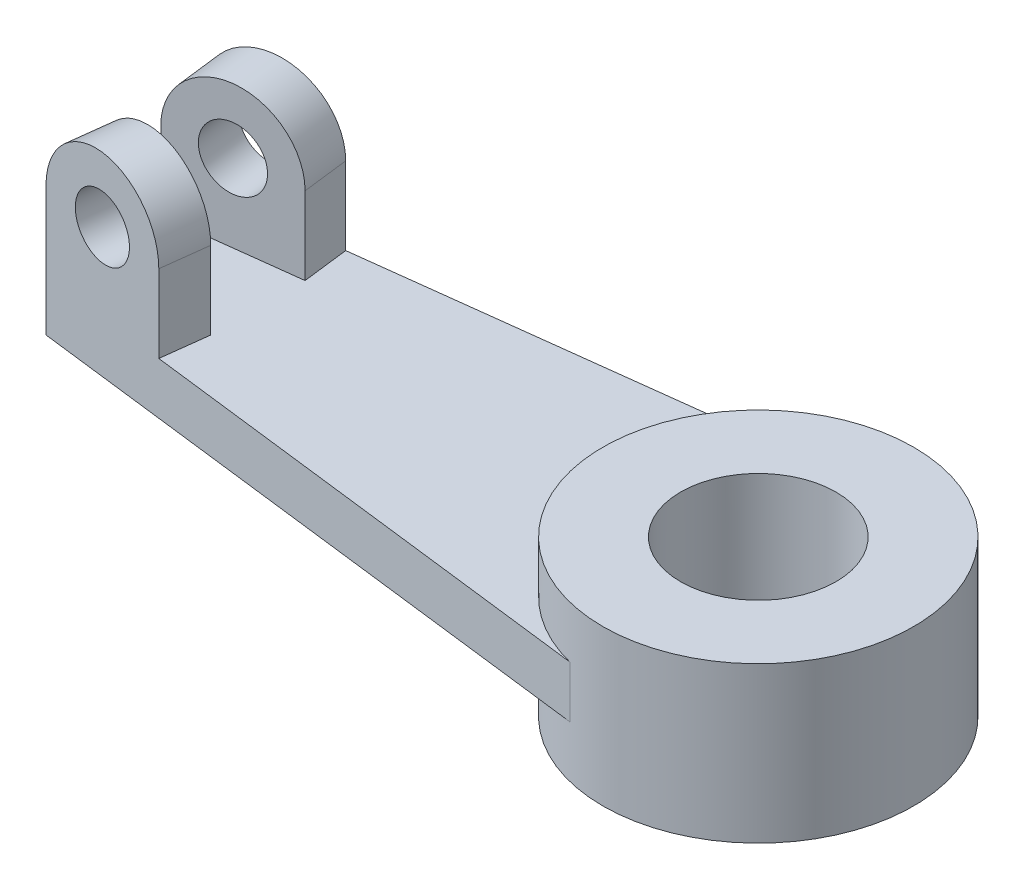
ISO-10303-21;
HEADER;
FILE_DESCRIPTION(('STEP AP214'),'2;1');
FILE_NAME('part.step','',(''),(''),'','','');
FILE_SCHEMA(('AUTOMOTIVE_DESIGN { 1 0 10303 214 1 1 1 1 }'));
ENDSEC;
DATA;
#1=APPLICATION_CONTEXT('core data for automotive mechanical design processes');
#2=APPLICATION_PROTOCOL_DEFINITION('international standard','automotive_design',2000,#1);
#3=PRODUCT_CONTEXT('',#1,'mechanical');
#4=PRODUCT('Part','Part','',(#3));
#5=PRODUCT_RELATED_PRODUCT_CATEGORY('part','',(#4));
#6=PRODUCT_DEFINITION_FORMATION('','',#4);
#7=PRODUCT_DEFINITION_CONTEXT('part definition',#1,'design');
#8=PRODUCT_DEFINITION('design','',#6,#7);
#9=PRODUCT_DEFINITION_SHAPE('','',#8);
#10=(LENGTH_UNIT() NAMED_UNIT(*) SI_UNIT(.MILLI.,.METRE.));
#11=(NAMED_UNIT(*) PLANE_ANGLE_UNIT() SI_UNIT($,.RADIAN.));
#12=(NAMED_UNIT(*) SI_UNIT($,.STERADIAN.) SOLID_ANGLE_UNIT());
#13=UNCERTAINTY_MEASURE_WITH_UNIT(LENGTH_MEASURE(1.E-05),#10,'distance_accuracy_value','');
#14=(GEOMETRIC_REPRESENTATION_CONTEXT(3) GLOBAL_UNCERTAINTY_ASSIGNED_CONTEXT((#13)) GLOBAL_UNIT_ASSIGNED_CONTEXT((#10,
#11,#12)) REPRESENTATION_CONTEXT('',''));
#15=CARTESIAN_POINT('',(0.,0.,0.));
#16=DIRECTION('',(0.,0.,1.));
#17=DIRECTION('',(1.,0.,0.));
#18=AXIS2_PLACEMENT_3D('',#15,#16,#17);
#19=CARTESIAN_POINT('',(0.,20.,0.));
#20=DIRECTION('',(0.,-1.,0.));
#21=DIRECTION('',(0.,0.,-1.));
#22=AXIS2_PLACEMENT_3D('',#19,#20,#21);
#23=CYLINDRICAL_SURFACE('',#22,30.);
#24=DIRECTION('',(0.,-1.,0.));
#25=VECTOR('',#24,1.);
#26=CARTESIAN_POINT('',(-7.23840787853918,10.,29.1136643414034));
#27=LINE('',#26,#25);
#28=CARTESIAN_POINT('',(-7.23840787853918,10.,29.1136643414034));
#29=VERTEX_POINT('',#28);
#30=CARTESIAN_POINT('',(-7.23840787853918,0.,29.1136643414034));
#31=VERTEX_POINT('',#30);
#32=EDGE_CURVE('E211',#29,#31,#27,.T.);
#33=ORIENTED_EDGE('',*,*,#32,.T.);
#34=CARTESIAN_POINT('',(0.,0.,0.));
#35=DIRECTION('',(0.,-1.,0.));
#36=DIRECTION('',(0.,0.,-1.));
#37=AXIS2_PLACEMENT_3D('',#34,#35,#36);
#38=CIRCLE('',#37,30.);
#39=CARTESIAN_POINT('',(-7.23840787853913,0.,-29.1136643414034));
#40=VERTEX_POINT('',#39);
#41=EDGE_CURVE('E187',#31,#40,#38,.T.);
#42=ORIENTED_EDGE('',*,*,#41,.T.);
#43=DIRECTION('',(0.,-1.,0.));
#44=VECTOR('',#43,1.);
#45=CARTESIAN_POINT('',(-7.23840787853913,10.,-29.1136643414034));
#46=LINE('',#45,#44);
#47=CARTESIAN_POINT('',(-7.23840787853913,10.,-29.1136643414034));
#48=VERTEX_POINT('',#47);
#49=EDGE_CURVE('E212',#48,#40,#46,.T.);
#50=ORIENTED_EDGE('',*,*,#49,.F.);
#51=CARTESIAN_POINT('',(0.,10.,0.));
#52=DIRECTION('',(0.,1.,0.));
#53=DIRECTION('',(0.,0.,1.));
#54=AXIS2_PLACEMENT_3D('',#51,#52,#53);
#55=CIRCLE('',#54,30.);
#56=EDGE_CURVE('E197',#48,#29,#55,.T.);
#57=ORIENTED_EDGE('',*,*,#56,.T.);
#58=EDGE_LOOP('',(#33,#42,#50,#57));
#59=FACE_BOUND('',#58,.T.);
#60=CARTESIAN_POINT('',(0.,20.,0.));
#61=DIRECTION('',(0.,1.,0.));
#62=DIRECTION('',(0.,0.,1.));
#63=AXIS2_PLACEMENT_3D('',#60,#61,#62);
#64=CIRCLE('',#63,30.);
#65=CARTESIAN_POINT('',(0.,20.,30.));
#66=VERTEX_POINT('',#65);
#67=EDGE_CURVE('E220',#66,#66,#64,.T.);
#68=ORIENTED_EDGE('',*,*,#67,.F.);
#69=EDGE_LOOP('',(#68));
#70=FACE_BOUND('',#69,.T.);
#71=CARTESIAN_POINT('',(0.,-10.,0.));
#72=DIRECTION('',(0.,-1.,0.));
#73=DIRECTION('',(0.,0.,-1.));
#74=AXIS2_PLACEMENT_3D('',#71,#72,#73);
#75=CIRCLE('',#74,30.);
#76=CARTESIAN_POINT('',(0.,-10.,-30.));
#77=VERTEX_POINT('',#76);
#78=EDGE_CURVE('E328',#77,#77,#75,.T.);
#79=ORIENTED_EDGE('',*,*,#78,.F.);
#80=EDGE_LOOP('',(#79));
#81=FACE_BOUND('',#80,.T.);
#82=ADVANCED_FACE('F43',(#59,#70,#81),#23,.T.);
#83=CARTESIAN_POINT('',(0.,0.,0.));
#84=DIRECTION('',(0.,1.,0.));
#85=DIRECTION('',(0.,0.,1.));
#86=AXIS2_PLACEMENT_3D('',#83,#84,#85);
#87=PLANE('',#86);
#88=DIRECTION('',(0.992586388695407,0.,-0.121541190452499));
#89=VECTOR('',#88,1.);
#90=CARTESIAN_POINT('',(-3.6192039392696,0.,-29.5568321707017));
#91=LINE('',#90,#89);
#92=CARTESIAN_POINT('',(-122.5,0.,-15.));
#93=VERTEX_POINT('',#92);
#94=EDGE_CURVE('E198',#93,#40,#91,.T.);
#95=ORIENTED_EDGE('',*,*,#94,.T.);
#96=ORIENTED_EDGE('',*,*,#41,.F.);
#97=DIRECTION('',(0.992586388695407,0.,0.121541190452499));
#98=VECTOR('',#97,1.);
#99=CARTESIAN_POINT('',(-3.61920393926959,0.,29.5568321707017));
#100=LINE('',#99,#98);
#101=CARTESIAN_POINT('',(-122.5,0.,15.));
#102=VERTEX_POINT('',#101);
#103=EDGE_CURVE('E207',#102,#31,#100,.T.);
#104=ORIENTED_EDGE('',*,*,#103,.F.);
#105=DIRECTION('',(0.,0.,-1.));
#106=VECTOR('',#105,1.);
#107=CARTESIAN_POINT('',(-122.5,0.,0.));
#108=LINE('',#107,#106);
#109=EDGE_CURVE('E192',#102,#93,#108,.T.);
#110=ORIENTED_EDGE('',*,*,#109,.T.);
#111=EDGE_LOOP('',(#95,#96,#104,#110));
#112=FACE_BOUND('',#111,.T.);
#113=ADVANCED_FACE('F261',(#112),#87,.F.);
#114=CARTESIAN_POINT('',(0.,20.,0.));
#115=DIRECTION('',(0.,1.,0.));
#116=DIRECTION('',(0.,0.,1.));
#117=AXIS2_PLACEMENT_3D('',#114,#115,#116);
#118=PLANE('',#117);
#119=CARTESIAN_POINT('',(0.,20.,0.));
#120=DIRECTION('',(0.,1.,0.));
#121=DIRECTION('',(0.,0.,1.));
#122=AXIS2_PLACEMENT_3D('',#119,#120,#121);
#123=CIRCLE('',#122,15.);
#124=CARTESIAN_POINT('',(0.,20.,15.));
#125=VERTEX_POINT('',#124);
#126=EDGE_CURVE('E322',#125,#125,#123,.T.);
#127=ORIENTED_EDGE('',*,*,#126,.F.);
#128=EDGE_LOOP('',(#127));
#129=FACE_BOUND('',#128,.T.);
#130=ORIENTED_EDGE('',*,*,#67,.T.);
#131=EDGE_LOOP('',(#130));
#132=FACE_BOUND('',#131,.T.);
#133=ADVANCED_FACE('F270',(#129,#132),#118,.T.);
#134=CARTESIAN_POINT('',(-122.5,10.,0.));
#135=DIRECTION('',(-1.,0.,0.));
#136=DIRECTION('',(0.,0.,1.));
#137=AXIS2_PLACEMENT_3D('',#134,#135,#136);
#138=PLANE('',#137);
#139=ORIENTED_EDGE('',*,*,#109,.F.);
#140=DIRECTION('',(0.,-1.,0.));
#141=VECTOR('',#140,1.);
#142=CARTESIAN_POINT('',(-122.5,10.,15.));
#143=LINE('',#142,#141);
#144=CARTESIAN_POINT('',(-122.5,10.,15.));
#145=VERTEX_POINT('',#144);
#146=EDGE_CURVE('E219',#145,#102,#143,.T.);
#147=ORIENTED_EDGE('',*,*,#146,.F.);
#148=DIRECTION('',(0.,0.,-1.));
#149=VECTOR('',#148,1.);
#150=CARTESIAN_POINT('',(-122.5,10.,0.));
#151=LINE('',#150,#149);
#152=CARTESIAN_POINT('',(-122.5,10.,-15.));
#153=VERTEX_POINT('',#152);
#154=EDGE_CURVE('E195',#145,#153,#151,.T.);
#155=ORIENTED_EDGE('',*,*,#154,.T.);
#156=DIRECTION('',(0.,-1.,0.));
#157=VECTOR('',#156,1.);
#158=CARTESIAN_POINT('',(-122.5,10.,-15.));
#159=LINE('',#158,#157);
#160=EDGE_CURVE('E203',#153,#93,#159,.T.);
#161=ORIENTED_EDGE('',*,*,#160,.T.);
#162=EDGE_LOOP('',(#139,#147,#155,#161));
#163=FACE_BOUND('',#162,.T.);
#164=ADVANCED_FACE('F255',(#163),#138,.T.);
#165=CARTESIAN_POINT('',(-3.61920393926959,10.,29.5568321707017));
#166=DIRECTION('',(0.121541190452499,0.,-0.992586388695407));
#167=DIRECTION('',(-0.992586388695407,0.,-0.121541190452499));
#168=AXIS2_PLACEMENT_3D('',#165,#166,#167);
#169=PLANE('',#168);
#170=ORIENTED_EDGE('',*,*,#103,.T.);
#171=ORIENTED_EDGE('',*,*,#32,.F.);
#172=DIRECTION('',(0.992586388695407,0.,0.121541190452499));
#173=VECTOR('',#172,1.);
#174=CARTESIAN_POINT('',(-3.61920393926959,10.,29.5568321707017));
#175=LINE('',#174,#173);
#176=CARTESIAN_POINT('',(-97.6853402826148,10.,18.0385297613125));
#177=VERTEX_POINT('',#176);
#178=EDGE_CURVE('E193',#177,#29,#175,.T.);
#179=ORIENTED_EDGE('',*,*,#178,.F.);
#180=DIRECTION('',(0.,-1.,0.));
#181=VECTOR('',#180,1.);
#182=CARTESIAN_POINT('',(-97.6853402826148,25.,18.0385297613125));
#183=LINE('',#182,#181);
#184=CARTESIAN_POINT('',(-97.6853402826148,25.,18.0385297613125));
#185=VERTEX_POINT('',#184);
#186=EDGE_CURVE('E137',#185,#177,#183,.T.);
#187=ORIENTED_EDGE('',*,*,#186,.F.);
#188=CARTESIAN_POINT('',(-110.092670141307,25.,16.5192648806562));
#189=DIRECTION('',(0.121541190452499,0.,-0.992586388695407));
#190=DIRECTION('',(-0.992586388695407,0.,-0.121541190452499));
#191=AXIS2_PLACEMENT_3D('',#188,#189,#190);
#192=CIRCLE('',#191,12.5);
#193=CARTESIAN_POINT('',(-122.5,25.,15.));
#194=VERTEX_POINT('',#193);
#195=EDGE_CURVE('E151',#194,#185,#192,.T.);
#196=ORIENTED_EDGE('',*,*,#195,.F.);
#197=DIRECTION('',(0.,1.,0.));
#198=VECTOR('',#197,1.);
#199=CARTESIAN_POINT('',(-122.5,0.,15.));
#200=LINE('',#199,#198);
#201=EDGE_CURVE('E145',#145,#194,#200,.T.);
#202=ORIENTED_EDGE('',*,*,#201,.F.);
#203=ORIENTED_EDGE('',*,*,#146,.T.);
#204=EDGE_LOOP('',(#170,#171,#179,#187,#196,#202,#203));
#205=FACE_BOUND('',#204,.T.);
#206=CARTESIAN_POINT('',(-110.092670141307,25.,16.5192648806562));
#207=DIRECTION('',(0.121541190452499,0.,-0.992586388695407));
#208=DIRECTION('',(-0.992586388695407,0.,-0.121541190452499));
#209=AXIS2_PLACEMENT_3D('',#206,#207,#208);
#210=CIRCLE('',#209,6.);
#211=CARTESIAN_POINT('',(-116.04818847348,25.,15.7900177379412));
#212=VERTEX_POINT('',#211);
#213=EDGE_CURVE('E332',#212,#212,#210,.T.);
#214=ORIENTED_EDGE('',*,*,#213,.T.);
#215=EDGE_LOOP('',(#214));
#216=FACE_BOUND('',#215,.T.);
#217=ADVANCED_FACE('F251',(#205,#216),#169,.F.);
#218=CARTESIAN_POINT('',(-3.6192039392696,10.,-29.5568321707017));
#219=DIRECTION('',(-0.121541190452499,0.,-0.992586388695407));
#220=DIRECTION('',(-0.992586388695407,0.,0.121541190452499));
#221=AXIS2_PLACEMENT_3D('',#218,#219,#220);
#222=PLANE('',#221);
#223=DIRECTION('',(0.,-1.,0.));
#224=VECTOR('',#223,1.);
#225=CARTESIAN_POINT('',(-97.6853402826148,25.,-18.0385297613125));
#226=LINE('',#225,#224);
#227=CARTESIAN_POINT('',(-97.6853402826148,25.,-18.0385297613125));
#228=VERTEX_POINT('',#227);
#229=CARTESIAN_POINT('',(-97.6853402826148,10.,-18.0385297613125));
#230=VERTEX_POINT('',#229);
#231=EDGE_CURVE('E63',#228,#230,#226,.T.);
#232=ORIENTED_EDGE('',*,*,#231,.T.);
#233=DIRECTION('',(0.992586388695407,0.,-0.121541190452499));
#234=VECTOR('',#233,1.);
#235=CARTESIAN_POINT('',(-3.6192039392696,10.,-29.5568321707017));
#236=LINE('',#235,#234);
#237=EDGE_CURVE('E202',#230,#48,#236,.T.);
#238=ORIENTED_EDGE('',*,*,#237,.T.);
#239=ORIENTED_EDGE('',*,*,#49,.T.);
#240=ORIENTED_EDGE('',*,*,#94,.F.);
#241=ORIENTED_EDGE('',*,*,#160,.F.);
#242=DIRECTION('',(0.,1.,0.));
#243=VECTOR('',#242,1.);
#244=CARTESIAN_POINT('',(-122.5,0.,-15.));
#245=LINE('',#244,#243);
#246=CARTESIAN_POINT('',(-122.5,25.,-15.));
#247=VERTEX_POINT('',#246);
#248=EDGE_CURVE('E166',#153,#247,#245,.T.);
#249=ORIENTED_EDGE('',*,*,#248,.T.);
#250=CARTESIAN_POINT('',(-110.092670141307,25.,-16.5192648806562));
#251=DIRECTION('',(-0.121541190452499,0.,-0.992586388695407));
#252=DIRECTION('',(-0.992586388695407,0.,0.121541190452499));
#253=AXIS2_PLACEMENT_3D('',#250,#251,#252);
#254=CIRCLE('',#253,12.5);
#255=EDGE_CURVE('E181',#247,#228,#254,.T.);
#256=ORIENTED_EDGE('',*,*,#255,.T.);
#257=EDGE_LOOP('',(#232,#238,#239,#240,#241,#249,#256));
#258=FACE_BOUND('',#257,.T.);
#259=CARTESIAN_POINT('',(-110.092670141307,25.,-16.5192648806562));
#260=DIRECTION('',(-0.121541190452499,0.,-0.992586388695407));
#261=DIRECTION('',(-0.992586388695407,0.,0.121541190452499));
#262=AXIS2_PLACEMENT_3D('',#259,#260,#261);
#263=CIRCLE('',#262,6.);
#264=CARTESIAN_POINT('',(-116.04818847348,25.,-15.7900177379412));
#265=VERTEX_POINT('',#264);
#266=EDGE_CURVE('E165',#265,#265,#263,.T.);
#267=ORIENTED_EDGE('',*,*,#266,.F.);
#268=EDGE_LOOP('',(#267));
#269=FACE_BOUND('',#268,.T.);
#270=ADVANCED_FACE('F246',(#258,#269),#222,.T.);
#271=CARTESIAN_POINT('',(0.,10.,0.));
#272=DIRECTION('',(0.,1.,0.));
#273=DIRECTION('',(0.,0.,1.));
#274=AXIS2_PLACEMENT_3D('',#271,#272,#273);
#275=PLANE('',#274);
#276=DIRECTION('',(-0.121541190452499,0.,0.992586388695407));
#277=VECTOR('',#276,1.);
#278=CARTESIAN_POINT('',(-94.0661363433452,10.,-11.5183024093892));
#279=LINE('',#278,#277);
#280=CARTESIAN_POINT('',(-96.5914695685423,10.,9.10525226305381));
#281=VERTEX_POINT('',#280);
#282=EDGE_CURVE('E60',#281,#177,#279,.T.);
#283=ORIENTED_EDGE('',*,*,#282,.T.);
#284=ORIENTED_EDGE('',*,*,#178,.T.);
#285=ORIENTED_EDGE('',*,*,#56,.F.);
#286=ORIENTED_EDGE('',*,*,#237,.F.);
#287=DIRECTION('',(-0.121541190452499,0.,-0.992586388695407));
#288=VECTOR('',#287,1.);
#289=CARTESIAN_POINT('',(-94.0661363433452,10.,11.5183024093892));
#290=LINE('',#289,#288);
#291=CARTESIAN_POINT('',(-96.5914695685423,10.,-9.10525226305381));
#292=VERTEX_POINT('',#291);
#293=EDGE_CURVE('E11',#292,#230,#290,.T.);
#294=ORIENTED_EDGE('',*,*,#293,.F.);
#295=DIRECTION('',(-0.992586388695407,0.,0.121541190452499));
#296=VECTOR('',#295,1.);
#297=CARTESIAN_POINT('',(-2.52533322519711,10.,-20.623554672443));
#298=LINE('',#297,#296);
#299=CARTESIAN_POINT('',(-121.406129285928,10.,-6.06672250174133));
#300=VERTEX_POINT('',#299);
#301=EDGE_CURVE('E225',#292,#300,#298,.T.);
#302=ORIENTED_EDGE('',*,*,#301,.T.);
#303=DIRECTION('',(0.121541190452499,0.,0.992586388695407));
#304=VECTOR('',#303,1.);
#305=CARTESIAN_POINT('',(-118.88079606073,10.,14.5568321707017));
#306=LINE('',#305,#304);
#307=EDGE_CURVE('E49',#153,#300,#306,.T.);
#308=ORIENTED_EDGE('',*,*,#307,.F.);
#309=ORIENTED_EDGE('',*,*,#154,.F.);
#310=DIRECTION('',(0.121541190452499,0.,-0.992586388695407));
#311=VECTOR('',#310,1.);
#312=CARTESIAN_POINT('',(-118.88079606073,10.,-14.5568321707017));
#313=LINE('',#312,#311);
#314=CARTESIAN_POINT('',(-121.406129285928,10.,6.06672250174133));
#315=VERTEX_POINT('',#314);
#316=EDGE_CURVE('E163',#145,#315,#313,.T.);
#317=ORIENTED_EDGE('',*,*,#316,.T.);
#318=DIRECTION('',(-0.992586388695407,0.,-0.121541190452499));
#319=VECTOR('',#318,1.);
#320=CARTESIAN_POINT('',(-2.52533322519711,10.,20.623554672443));
#321=LINE('',#320,#319);
#322=EDGE_CURVE('E132',#281,#315,#321,.T.);
#323=ORIENTED_EDGE('',*,*,#322,.F.);
#324=EDGE_LOOP('',(#283,#284,#285,#286,#294,#302,#308,#309,#317,#323));
#325=FACE_BOUND('',#324,.T.);
#326=ADVANCED_FACE('F238',(#325),#275,.T.);
#327=CARTESIAN_POINT('',(-96.5914695685423,25.,-9.10525226305381));
#328=DIRECTION('',(0.992586388695407,0.,-0.121541190452499));
#329=DIRECTION('',(-0.121541190452499,0.,-0.992586388695407));
#330=AXIS2_PLACEMENT_3D('',#327,#328,#329);
#331=PLANE('',#330);
#332=DIRECTION('',(0.,-1.,0.));
#333=VECTOR('',#332,1.);
#334=CARTESIAN_POINT('',(-96.5914695685423,25.,-9.10525226305381));
#335=LINE('',#334,#333);
#336=CARTESIAN_POINT('',(-96.5914695685423,25.,-9.10525226305381));
#337=VERTEX_POINT('',#336);
#338=EDGE_CURVE('E176',#337,#292,#335,.T.);
#339=ORIENTED_EDGE('',*,*,#338,.T.);
#340=ORIENTED_EDGE('',*,*,#293,.T.);
#341=ORIENTED_EDGE('',*,*,#231,.F.);
#342=DIRECTION('',(-0.121541190452499,0.,-0.992586388695407));
#343=VECTOR('',#342,1.);
#344=CARTESIAN_POINT('',(-96.5914695685423,25.,-9.10525226305381));
#345=LINE('',#344,#343);
#346=EDGE_CURVE('E183',#337,#228,#345,.T.);
#347=ORIENTED_EDGE('',*,*,#346,.F.);
#348=EDGE_LOOP('',(#339,#340,#341,#347));
#349=FACE_BOUND('',#348,.T.);
#350=ADVANCED_FACE('F245',(#349),#331,.T.);
#351=CARTESIAN_POINT('',(-108.998799427235,25.,-7.58598738239757));
#352=DIRECTION('',(-0.121541190452499,0.,-0.992586388695407));
#353=DIRECTION('',(-0.992586388695407,0.,0.121541190452499));
#354=AXIS2_PLACEMENT_3D('',#351,#352,#353);
#355=CYLINDRICAL_SURFACE('',#354,12.5);
#356=ORIENTED_EDGE('',*,*,#255,.F.);
#357=DIRECTION('',(-0.121541190452499,0.,-0.992586388695407));
#358=VECTOR('',#357,1.);
#359=CARTESIAN_POINT('',(-121.406129285928,25.,-6.06672250174133));
#360=LINE('',#359,#358);
#361=CARTESIAN_POINT('',(-121.406129285928,25.,-6.06672250174133));
#362=VERTEX_POINT('',#361);
#363=EDGE_CURVE('E177',#362,#247,#360,.T.);
#364=ORIENTED_EDGE('',*,*,#363,.F.);
#365=CARTESIAN_POINT('',(-108.998799427235,25.,-7.58598738239757));
#366=DIRECTION('',(-0.121541190452499,0.,-0.992586388695407));
#367=DIRECTION('',(-0.992586388695407,0.,0.121541190452499));
#368=AXIS2_PLACEMENT_3D('',#365,#366,#367);
#369=CIRCLE('',#368,12.5);
#370=EDGE_CURVE('E173',#362,#337,#369,.T.);
#371=ORIENTED_EDGE('',*,*,#370,.T.);
#372=ORIENTED_EDGE('',*,*,#346,.T.);
#373=EDGE_LOOP('',(#356,#364,#371,#372));
#374=FACE_BOUND('',#373,.T.);
#375=ADVANCED_FACE('F244',(#374),#355,.T.);
#376=CARTESIAN_POINT('',(-121.406129285928,0.,-6.06672250174133));
#377=DIRECTION('',(-0.992586388695407,0.,0.121541190452499));
#378=DIRECTION('',(0.121541190452499,0.,0.992586388695407));
#379=AXIS2_PLACEMENT_3D('',#376,#377,#378);
#380=PLANE('',#379);
#381=ORIENTED_EDGE('',*,*,#248,.F.);
#382=ORIENTED_EDGE('',*,*,#307,.T.);
#383=DIRECTION('',(0.,1.,0.));
#384=VECTOR('',#383,1.);
#385=CARTESIAN_POINT('',(-121.406129285928,0.,-6.06672250174133));
#386=LINE('',#385,#384);
#387=EDGE_CURVE('E171',#300,#362,#386,.T.);
#388=ORIENTED_EDGE('',*,*,#387,.T.);
#389=ORIENTED_EDGE('',*,*,#363,.T.);
#390=EDGE_LOOP('',(#381,#382,#388,#389));
#391=FACE_BOUND('',#390,.T.);
#392=ADVANCED_FACE('F227',(#391),#380,.T.);
#393=CARTESIAN_POINT('',(-108.998799427235,25.,-7.58598738239757));
#394=DIRECTION('',(-0.121541190452499,0.,-0.992586388695407));
#395=DIRECTION('',(-0.992586388695407,0.,0.121541190452499));
#396=AXIS2_PLACEMENT_3D('',#393,#394,#395);
#397=PLANE('',#396);
#398=ORIENTED_EDGE('',*,*,#301,.F.);
#399=ORIENTED_EDGE('',*,*,#338,.F.);
#400=ORIENTED_EDGE('',*,*,#370,.F.);
#401=ORIENTED_EDGE('',*,*,#387,.F.);
#402=EDGE_LOOP('',(#398,#399,#400,#401));
#403=FACE_BOUND('',#402,.T.);
#404=CARTESIAN_POINT('',(-108.998799427235,25.,-7.58598738239757));
#405=DIRECTION('',(-0.121541190452499,0.,-0.992586388695407));
#406=DIRECTION('',(-0.992586388695407,0.,0.121541190452499));
#407=AXIS2_PLACEMENT_3D('',#404,#405,#406);
#408=CIRCLE('',#407,6.);
#409=CARTESIAN_POINT('',(-114.954317759407,25.,-6.85674023968258));
#410=VERTEX_POINT('',#409);
#411=EDGE_CURVE('E164',#410,#410,#408,.T.);
#412=ORIENTED_EDGE('',*,*,#411,.T.);
#413=EDGE_LOOP('',(#412));
#414=FACE_BOUND('',#413,.T.);
#415=ADVANCED_FACE('F234',(#403,#414),#397,.F.);
#416=CARTESIAN_POINT('',(-108.998799427235,25.,-7.58598738239757));
#417=DIRECTION('',(-0.121541190452499,0.,-0.992586388695407));
#418=DIRECTION('',(-0.992586388695407,0.,0.121541190452499));
#419=AXIS2_PLACEMENT_3D('',#416,#417,#418);
#420=CYLINDRICAL_SURFACE('',#419,6.);
#421=ORIENTED_EDGE('',*,*,#411,.F.);
#422=EDGE_LOOP('',(#421));
#423=FACE_BOUND('',#422,.T.);
#424=ORIENTED_EDGE('',*,*,#266,.T.);
#425=EDGE_LOOP('',(#424));
#426=FACE_BOUND('',#425,.T.);
#427=ADVANCED_FACE('F291',(#423,#426),#420,.F.);
#428=CARTESIAN_POINT('',(-96.5914695685423,25.,9.10525226305381));
#429=DIRECTION('',(0.992586388695407,0.,0.121541190452499));
#430=DIRECTION('',(-0.121541190452499,0.,0.992586388695407));
#431=AXIS2_PLACEMENT_3D('',#428,#429,#430);
#432=PLANE('',#431);
#433=DIRECTION('',(0.,-1.,0.));
#434=VECTOR('',#433,1.);
#435=CARTESIAN_POINT('',(-96.5914695685423,25.,9.10525226305381));
#436=LINE('',#435,#434);
#437=CARTESIAN_POINT('',(-96.5914695685423,25.,9.10525226305381));
#438=VERTEX_POINT('',#437);
#439=EDGE_CURVE('E150',#438,#281,#436,.T.);
#440=ORIENTED_EDGE('',*,*,#439,.F.);
#441=DIRECTION('',(-0.121541190452499,0.,0.992586388695407));
#442=VECTOR('',#441,1.);
#443=CARTESIAN_POINT('',(-96.5914695685423,25.,9.10525226305381));
#444=LINE('',#443,#442);
#445=EDGE_CURVE('E147',#438,#185,#444,.T.);
#446=ORIENTED_EDGE('',*,*,#445,.T.);
#447=ORIENTED_EDGE('',*,*,#186,.T.);
#448=ORIENTED_EDGE('',*,*,#282,.F.);
#449=EDGE_LOOP('',(#440,#446,#447,#448));
#450=FACE_BOUND('',#449,.T.);
#451=ADVANCED_FACE('F258',(#450),#432,.T.);
#452=CARTESIAN_POINT('',(-108.998799427235,25.,7.58598738239757));
#453=DIRECTION('',(-0.121541190452499,0.,0.992586388695407));
#454=DIRECTION('',(-0.992586388695407,0.,-0.121541190452499));
#455=AXIS2_PLACEMENT_3D('',#452,#453,#454);
#456=CYLINDRICAL_SURFACE('',#455,12.5);
#457=ORIENTED_EDGE('',*,*,#195,.T.);
#458=ORIENTED_EDGE('',*,*,#445,.F.);
#459=CARTESIAN_POINT('',(-108.998799427235,25.,7.58598738239757));
#460=DIRECTION('',(0.121541190452499,0.,-0.992586388695407));
#461=DIRECTION('',(-0.992586388695407,0.,-0.121541190452499));
#462=AXIS2_PLACEMENT_3D('',#459,#460,#461);
#463=CIRCLE('',#462,12.5);
#464=CARTESIAN_POINT('',(-121.406129285928,25.,6.06672250174133));
#465=VERTEX_POINT('',#464);
#466=EDGE_CURVE('E128',#465,#438,#463,.T.);
#467=ORIENTED_EDGE('',*,*,#466,.F.);
#468=DIRECTION('',(-0.121541190452499,0.,0.992586388695407));
#469=VECTOR('',#468,1.);
#470=CARTESIAN_POINT('',(-121.406129285928,25.,6.06672250174133));
#471=LINE('',#470,#469);
#472=EDGE_CURVE('E139',#465,#194,#471,.T.);
#473=ORIENTED_EDGE('',*,*,#472,.T.);
#474=EDGE_LOOP('',(#457,#458,#467,#473));
#475=FACE_BOUND('',#474,.T.);
#476=ADVANCED_FACE('F146',(#475),#456,.T.);
#477=CARTESIAN_POINT('',(-121.406129285928,0.,6.06672250174133));
#478=DIRECTION('',(-0.992586388695407,0.,-0.121541190452499));
#479=DIRECTION('',(0.121541190452499,0.,-0.992586388695407));
#480=AXIS2_PLACEMENT_3D('',#477,#478,#479);
#481=PLANE('',#480);
#482=ORIENTED_EDGE('',*,*,#201,.T.);
#483=ORIENTED_EDGE('',*,*,#472,.F.);
#484=DIRECTION('',(0.,1.,0.));
#485=VECTOR('',#484,1.);
#486=CARTESIAN_POINT('',(-121.406129285928,0.,6.06672250174133));
#487=LINE('',#486,#485);
#488=EDGE_CURVE('E123',#315,#465,#487,.T.);
#489=ORIENTED_EDGE('',*,*,#488,.F.);
#490=ORIENTED_EDGE('',*,*,#316,.F.);
#491=EDGE_LOOP('',(#482,#483,#489,#490));
#492=FACE_BOUND('',#491,.T.);
#493=ADVANCED_FACE('F136',(#492),#481,.T.);
#494=CARTESIAN_POINT('',(-108.998799427235,25.,7.58598738239757));
#495=DIRECTION('',(-0.121541190452499,0.,0.992586388695407));
#496=DIRECTION('',(-0.992586388695407,0.,-0.121541190452499));
#497=AXIS2_PLACEMENT_3D('',#494,#495,#496);
#498=PLANE('',#497);
#499=ORIENTED_EDGE('',*,*,#322,.T.);
#500=ORIENTED_EDGE('',*,*,#488,.T.);
#501=ORIENTED_EDGE('',*,*,#466,.T.);
#502=ORIENTED_EDGE('',*,*,#439,.T.);
#503=EDGE_LOOP('',(#499,#500,#501,#502));
#504=FACE_BOUND('',#503,.T.);
#505=CARTESIAN_POINT('',(-108.998799427235,25.,7.58598738239757));
#506=DIRECTION('',(0.121541190452499,0.,-0.992586388695407));
#507=DIRECTION('',(-0.992586388695407,0.,-0.121541190452499));
#508=AXIS2_PLACEMENT_3D('',#505,#506,#507);
#509=CIRCLE('',#508,6.);
#510=CARTESIAN_POINT('',(-114.954317759407,25.,6.85674023968258));
#511=VERTEX_POINT('',#510);
#512=EDGE_CURVE('E157',#511,#511,#509,.T.);
#513=ORIENTED_EDGE('',*,*,#512,.F.);
#514=EDGE_LOOP('',(#513));
#515=FACE_BOUND('',#514,.T.);
#516=ADVANCED_FACE('F130',(#504,#515),#498,.F.);
#517=CARTESIAN_POINT('',(-108.998799427235,25.,7.58598738239757));
#518=DIRECTION('',(-0.121541190452499,0.,0.992586388695407));
#519=DIRECTION('',(-0.992586388695407,0.,-0.121541190452499));
#520=AXIS2_PLACEMENT_3D('',#517,#518,#519);
#521=CYLINDRICAL_SURFACE('',#520,6.);
#522=ORIENTED_EDGE('',*,*,#512,.T.);
#523=EDGE_LOOP('',(#522));
#524=FACE_BOUND('',#523,.T.);
#525=ORIENTED_EDGE('',*,*,#213,.F.);
#526=EDGE_LOOP('',(#525));
#527=FACE_BOUND('',#526,.T.);
#528=ADVANCED_FACE('F304',(#524,#527),#521,.F.);
#529=CARTESIAN_POINT('',(0.,-10.,0.));
#530=DIRECTION('',(0.,-1.,0.));
#531=DIRECTION('',(0.,0.,-1.));
#532=AXIS2_PLACEMENT_3D('',#529,#530,#531);
#533=PLANE('',#532);
#534=CARTESIAN_POINT('',(0.,-10.,0.));
#535=DIRECTION('',(0.,-1.,0.));
#536=DIRECTION('',(0.,0.,-1.));
#537=AXIS2_PLACEMENT_3D('',#534,#535,#536);
#538=CIRCLE('',#537,15.);
#539=CARTESIAN_POINT('',(0.,-10.,-15.));
#540=VERTEX_POINT('',#539);
#541=EDGE_CURVE('E321',#540,#540,#538,.T.);
#542=ORIENTED_EDGE('',*,*,#541,.F.);
#543=EDGE_LOOP('',(#542));
#544=FACE_BOUND('',#543,.T.);
#545=ORIENTED_EDGE('',*,*,#78,.T.);
#546=EDGE_LOOP('',(#545));
#547=FACE_BOUND('',#546,.T.);
#548=ADVANCED_FACE('F308',(#544,#547),#533,.T.);
#549=CARTESIAN_POINT('',(0.,36.,0.));
#550=DIRECTION('',(0.,-1.,0.));
#551=DIRECTION('',(0.,0.,-1.));
#552=AXIS2_PLACEMENT_3D('',#549,#550,#551);
#553=CYLINDRICAL_SURFACE('',#552,15.);
#554=ORIENTED_EDGE('',*,*,#126,.T.);
#555=EDGE_LOOP('',(#554));
#556=FACE_BOUND('',#555,.T.);
#557=ORIENTED_EDGE('',*,*,#541,.T.);
#558=EDGE_LOOP('',(#557));
#559=FACE_BOUND('',#558,.T.);
#560=ADVANCED_FACE('F315',(#556,#559),#553,.F.);
#561=CLOSED_SHELL('',(#82,#113,#133,#164,#217,#270,#326,#350,#375,#392,#415,#427,#451,#476,#493,
#516,#528,#548,#560));
#562=MANIFOLD_SOLID_BREP('B2',#561);
#563=ADVANCED_BREP_SHAPE_REPRESENTATION('',(#18,#562),#14);
#564=SHAPE_DEFINITION_REPRESENTATION(#9,#563);
ENDSEC;
END-ISO-10303-21;
